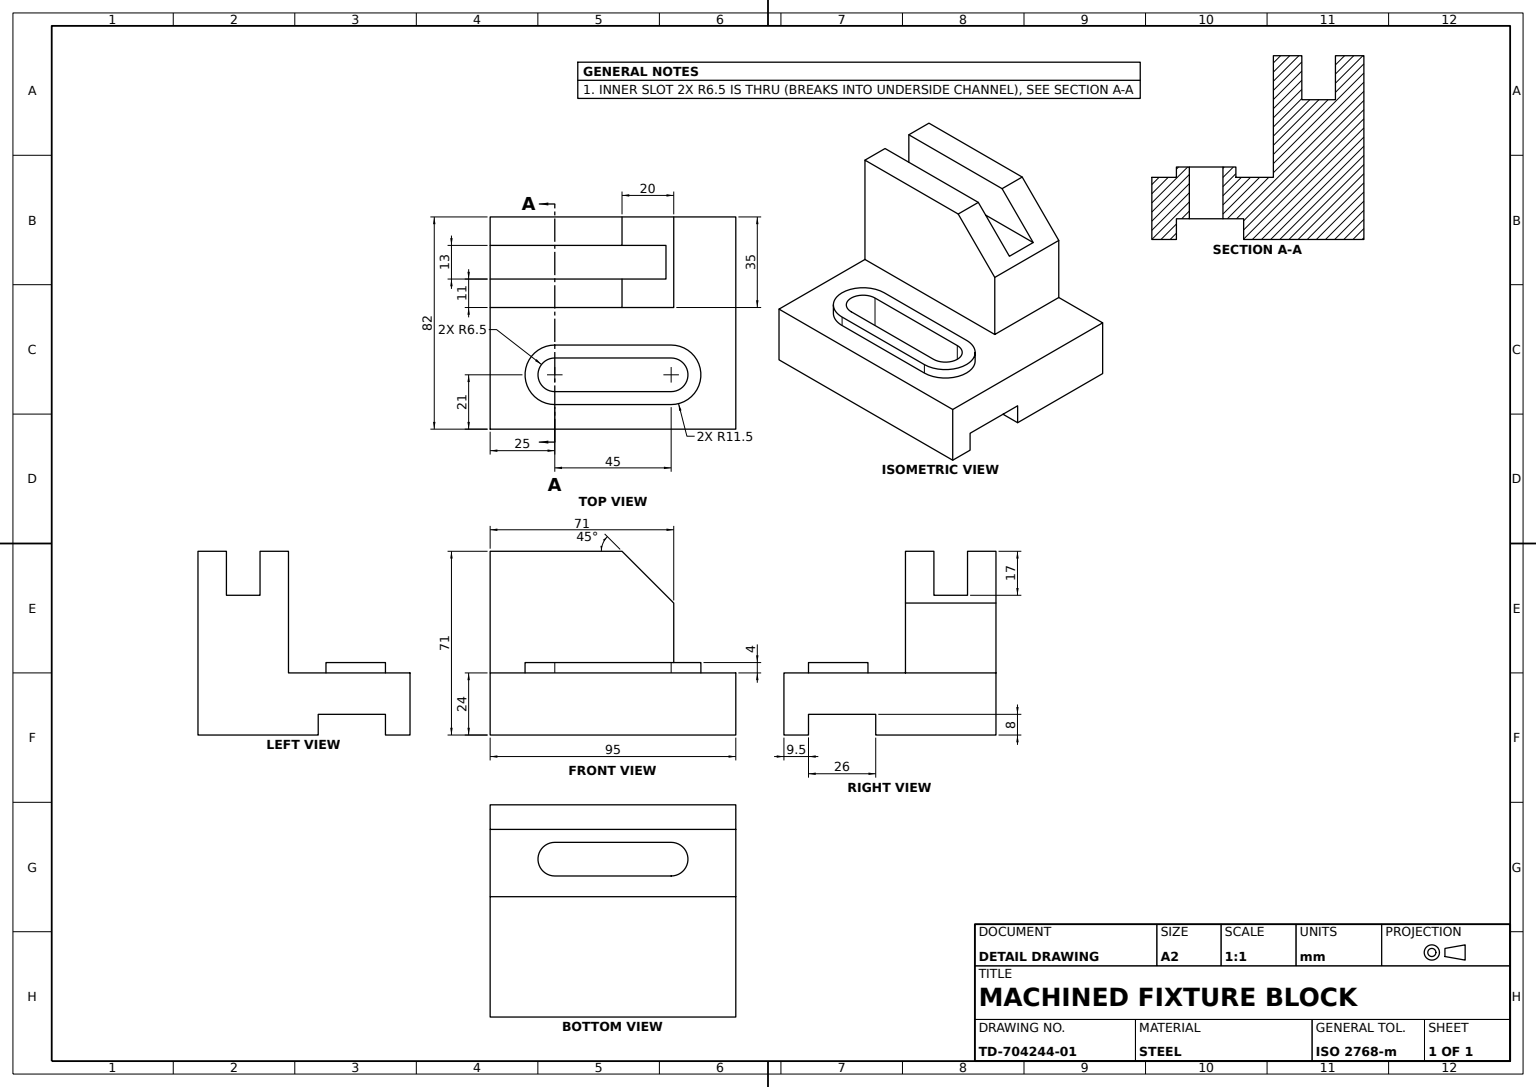
from build123d import *

# Parameters (mm, degrees)
BASE_BLOCK_DEPTH           = 95
UPRIGHT_BLOCK_DEPTH        = 71
UPRIGHT_CHAMFER_20X45_SIZE = 20
SLOT_RIM_BOSS_DEPTH        = 4
THROUGH_START              = -154
THROUGH_SLOT_CUT_DEPTH     = 154


with BuildPart() as part:
    # Base and Upright Profile Sketch → Base Block (new body)
    with BuildSketch(Plane(origin=(0, 0, 0), x_dir=(0, 0, -1), z_dir=(1, 0, 0))):
        Polygon((35.5, 0), (35.5, 8), (9.5, 8), (9.5, 0), (0, 0), (0, 24), (82, 24), (82, 0), align=None)
    extrude(amount=BASE_BLOCK_DEPTH)

    # Sketch1_3 → Upright Block (add)
    with BuildSketch(Plane(origin=(0, 0, 0), x_dir=(0, 0, -1), z_dir=(1, 0, 0))):
        Polygon((58, 54), (58, 71), (47, 71), (47, 24), (82, 24), (82, 71), (71, 71), (71, 54), align=None)
    extrude(amount=UPRIGHT_BLOCK_DEPTH)

    # Upright Chamfer 20x45
    upright_chamfer_20x45_edges = [part.edges().sort_by_distance(p)[0] for p in [
        (71, 71, -52.5),
    ]]
    chamfer(upright_chamfer_20x45_edges, length=UPRIGHT_CHAMFER_20X45_SIZE)

    # Slot Rim Sketch → Slot Rim Boss (add)
    with BuildSketch(Plane(origin=(0, 24, 0), x_dir=(1, 0, 0), z_dir=(0, 1, 0))):
        with BuildLine():
            Line((25, 32.5), (70, 32.5))
            ThreePointArc((70, 32.5), (81.5, 21), (70, 9.5))
            Line((70, 9.5), (25, 9.5))
            ThreePointArc((25, 9.5), (13.5, 21), (25, 32.5))
        make_face()
        with BuildLine():
            Line((25, 27.5), (70, 27.5))
            ThreePointArc((70, 27.5), (76.5, 21), (70, 14.5))
            Line((70, 14.5), (25, 14.5))
            ThreePointArc((25, 14.5), (18.5, 21), (25, 27.5))
        make_face(mode=Mode.SUBTRACT)
    extrude(amount=SLOT_RIM_BOSS_DEPTH)

    # Through Slot Sketch → Through Slot Cut (cut)
    with BuildSketch(Plane(origin=(0, 24, 0), x_dir=(1, 0, 0), z_dir=(0, 1, 0)).offset(THROUGH_START)):
        with BuildLine():
            Line((25, 27.5), (70, 27.5))
            ThreePointArc((70, 27.5), (76.5, 21), (70, 14.5))
            Line((70, 14.5), (25, 14.5))
            ThreePointArc((25, 14.5), (18.5, 21), (25, 27.5))
        make_face()
    extrude(amount=THROUGH_SLOT_CUT_DEPTH, mode=Mode.SUBTRACT)


solid = part.part
